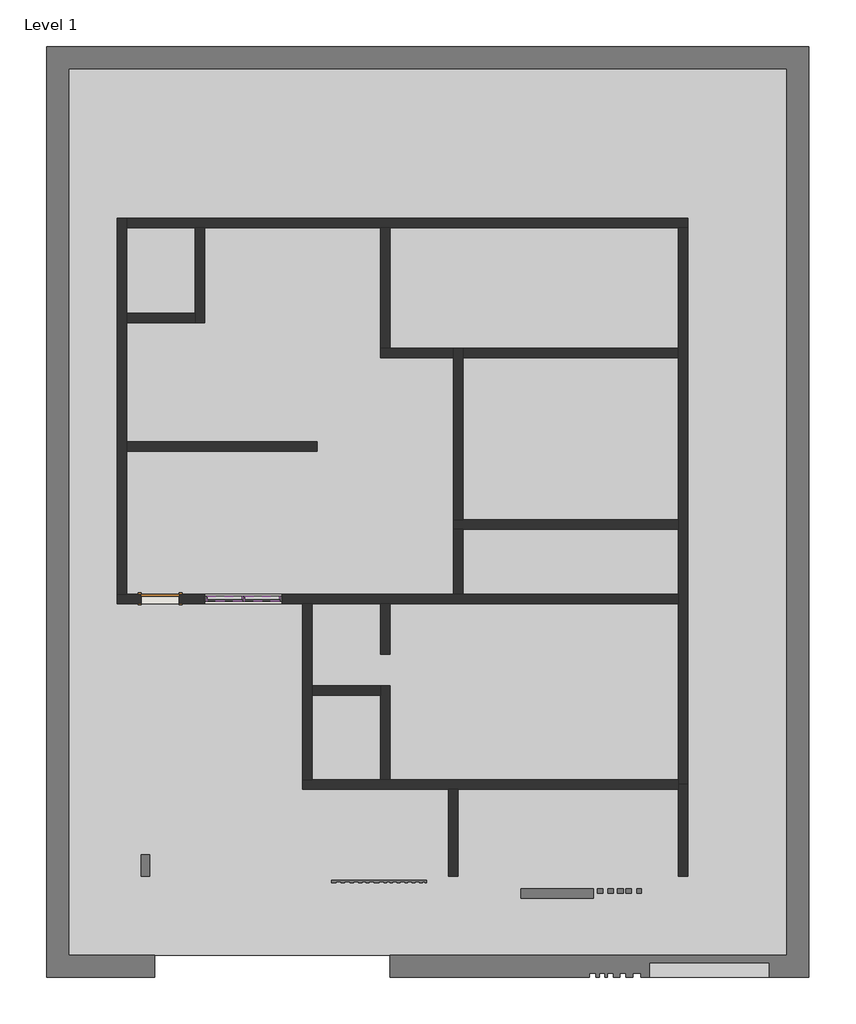
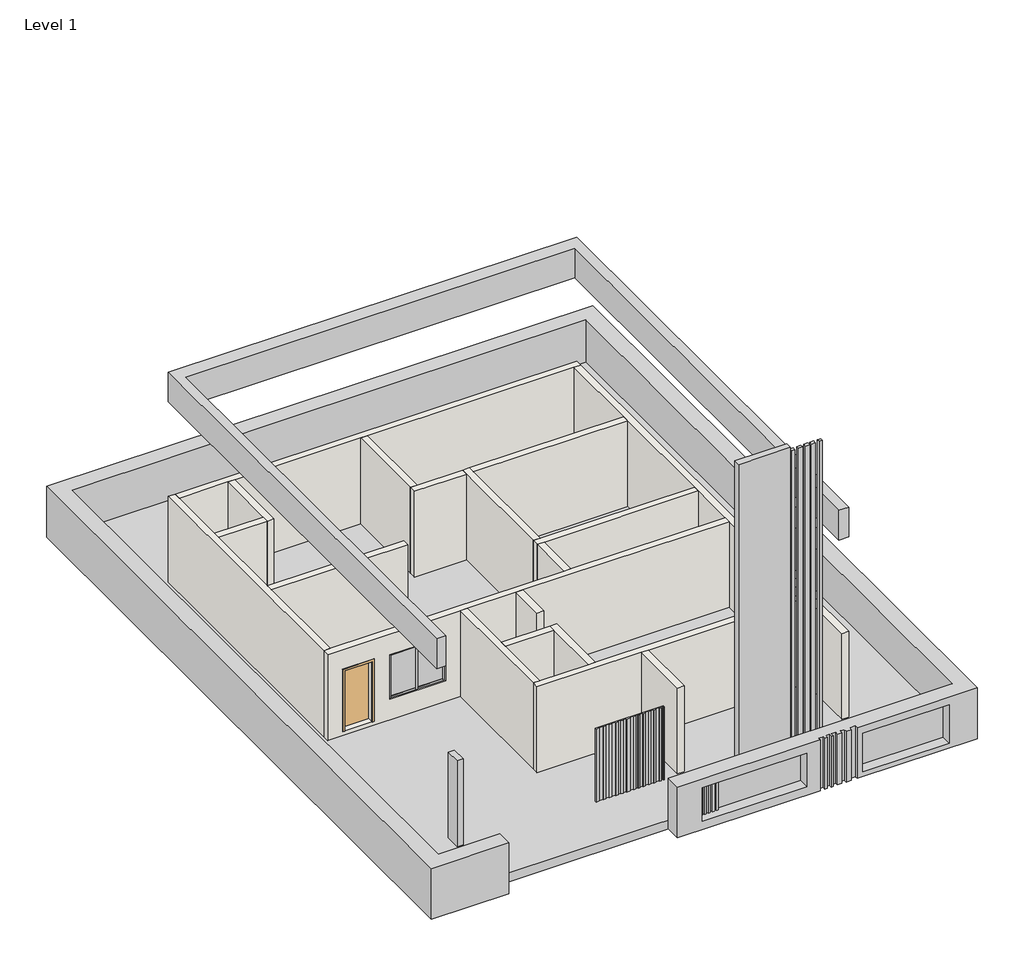
# One storey: 20 walls, 7 members, 3 proxies, 2 plates, 1 door.
"""IFC4 building model written with IfcOpenShell, lengths in millimetres."""

from ifc_helpers import new_model, si_unit, origin, origin_with_axes, place, context, project, spatial, polyline, outline, extrude, faceted_brep, transform, mapped, element, save
from components import generic_models_1_generic_models_1_f562e270, generic_models_2_generic_models_2_9e54925f, generic_models_3_generic_models_3_60b2bde9, door_a90ba1ad, member_86adc6a2, member_ef177d9f, member_d616553b, system_panel_glazed_f96bbed7

model = new_model("IFC4")

# Units and contexts
model_context = context("Model", 3, world=origin())
ifc_project = project(units=[si_unit("LENGTHUNIT", "METRE", prefix="MILLI")], contexts=[model_context])

# Site, building, storey
site = spatial("IfcSite", under=ifc_project)
building = spatial("IfcBuilding", under=site)
storey = spatial("IfcBuildingStorey", under=building, Name="Level 1", Elevation=0.0)

# Proxies
placement = place(None, origin())
generic_models_1_generic_models_1_shape = generic_models_1_generic_models_1_f562e270(model_context)
element("IfcBuildingElementProxy", 1, Name="Generic Models 1 : Generic Models 1", ObjectType="Generic Models 1 : Generic Models 1", at=placement, inside=storey, context=model_context, shape_type="MappedRepresentation", body=[
    mapped(generic_models_1_generic_models_1_shape, transform((0.0, 0.0, 0.0), x_axis=(1.0, 0.0, 0.0), y_axis=(0.0, 1.0, 0.0), z_axis=(0.0, 0.0, 1.0))),
])
generic_models_2_generic_models_2_shape = generic_models_2_generic_models_2_9e54925f(model_context)
element("IfcBuildingElementProxy", 2, Name="Generic Models 2 : Generic Models 2", ObjectType="Generic Models 2 : Generic Models 2", at=placement, inside=storey, context=model_context, shape_type="MappedRepresentation", body=[
    mapped(generic_models_2_generic_models_2_shape, transform((0.0, 0.0, 0.0), x_axis=(1.0, 0.0, 0.0), y_axis=(0.0, 1.0, 0.0), z_axis=(0.0, 0.0, 1.0))),
])
generic_models_3_generic_models_3_shape = generic_models_3_generic_models_3_60b2bde9(model_context)
element("IfcBuildingElementProxy", 3, Name="Generic Models 3 : Generic Models 3", ObjectType="Generic Models 3 : Generic Models 3", at=placement, inside=storey, context=model_context, shape_type="MappedRepresentation", body=[
    mapped(generic_models_3_generic_models_3_shape, transform((0.0, 0.0, 0.0), x_axis=(1.0, 0.0, 0.0), y_axis=(0.0, 1.0, 0.0), z_axis=(0.0, 0.0, 1.0))),
])

# Door
door_shape = door_a90ba1ad(model_context)
element("IfcDoor", 4, ObjectType="Single-Flush : 36\" x 84\"", at=placement, inside=storey, context=model_context, shape_type="MappedRepresentation", body=[
    mapped(door_shape, transform((-16900.3047537, -14441.5428796, 152.4), x_axis=(-1.0, 0.0, 0.0), y_axis=(0.0, -1.0, 0.0), z_axis=(0.0, 0.0, 1.0))),
])

# Members
member_shape = member_86adc6a2(model_context)
element("IfcMember", 5, ObjectType="Rectangular Mullion : 2.5\" x 5\" rectangular", at=placement, inside=storey, context=model_context, shape_type="MappedRepresentation", body=[
    mapped(member_shape, transform((-14868.3047537, -14441.5428796, 2302.9490585), x_axis=(0.0, 0.0, 1.0), y_axis=(0.0, 1.0, 0.0), z_axis=(-1.0, 0.0, 0.0))),
])
element("IfcMember", 6, ObjectType="Rectangular Mullion : 2.5\" x 5\" rectangular", at=placement, inside=storey, context=model_context, shape_type="MappedRepresentation", body=[
    mapped(member_shape, transform((-15770.0047537, -14441.5428796, 2302.9490585), x_axis=(0.0, 0.0, 1.0), y_axis=(0.0, 1.0, 0.0), z_axis=(-1.0, 0.0, 0.0))),
])
member_2_shape = member_ef177d9f(model_context)
element("IfcMember", 7, ObjectType="Rectangular Mullion : 2.5\" x 5\" rectangular", at=placement, inside=storey, context=model_context, shape_type="MappedRepresentation", body=[
    mapped(member_2_shape, transform((-14900.0547537, -14441.5428796, 726.5200737), x_axis=(-1.0, 0.0, 0.0), y_axis=(0.0, 1.0, 0.0), z_axis=(0.0, 0.0, -1.0))),
])
element("IfcMember", 8, ObjectType="Rectangular Mullion : 2.5\" x 5\" rectangular", at=placement, inside=storey, context=model_context, shape_type="MappedRepresentation", body=[
    mapped(member_shape, transform((-14931.8047537, -14441.5428796, 726.5200737), x_axis=(0.0, 0.0, -1.0), y_axis=(0.0, 1.0, 0.0), z_axis=(1.0, 0.0, 0.0))),
])
element("IfcMember", 9, ObjectType="Rectangular Mullion : 2.5\" x 5\" rectangular", at=placement, inside=storey, context=model_context, shape_type="MappedRepresentation", body=[
    mapped(member_shape, transform((-14030.1047537, -14441.5428796, 726.5200737), x_axis=(0.0, 0.0, -1.0), y_axis=(0.0, 1.0, 0.0), z_axis=(1.0, 0.0, 0.0))),
])
member_3_shape = member_d616553b(model_context)
element("IfcMember", 10, ObjectType="Rectangular Mullion : 2.5\" x 5\" rectangular", at=placement, inside=storey, context=model_context, shape_type="MappedRepresentation", body=[
    mapped(member_3_shape, transform((-13966.6047537, -14441.5428796, 2302.9490585), x_axis=(1.0, 0.0, 0.0), y_axis=(0.0, 1.0, 0.0), z_axis=(0.0, 0.0, 1.0))),
])
element("IfcMember", 11, ObjectType="Rectangular Mullion : 2.5\" x 5\" rectangular", at=placement, inside=storey, context=model_context, shape_type="MappedRepresentation", body=[
    mapped(member_3_shape, transform((-15833.5047537, -14441.5428796, 726.5200737), x_axis=(-1.0, 0.0, 0.0), y_axis=(0.0, 1.0, 0.0), z_axis=(0.0, 0.0, -1.0))),
])

# Plates
system_panel_glazed_shape = system_panel_glazed_f96bbed7(model_context)
element("IfcPlate", 12, ObjectType="System Panel : Glazed", at=placement, inside=storey, context=model_context, shape_type="MappedRepresentation", body=[
    mapped(system_panel_glazed_shape, transform((-14449.2047537, -14441.5428796, 790.0200737), x_axis=(-1.0, 0.0, 0.0), y_axis=(0.0, -1.0, 0.0), z_axis=(0.0, 0.0, 1.0))),
])
element("IfcPlate", 13, ObjectType="System Panel : Glazed", at=placement, inside=storey, context=model_context, shape_type="MappedRepresentation", body=[
    mapped(system_panel_glazed_shape, transform((-15350.9047537, -14441.5428796, 790.0200737), x_axis=(-1.0, 0.0, 0.0), y_axis=(0.0, -1.0, 0.0), z_axis=(0.0, 0.0, 1.0))),
])

# Walls
element("IfcWall", 14, ObjectType="9\"", at=placement, inside=storey, context=model_context, shape_type="Brep", body=[
    faceted_brep([(-17929.0047537, -14555.8428796, 0.0), (-13471.3047537, -14555.8428796, 0.0), (-13242.7047537, -14555.8428796, 0.0), (-11604.4047537, -14555.8428796, 0.0), (-11375.8047537, -14555.8428796, 0.0), (-4441.6047537, -14555.8428796, 0.0), (-4441.6047537, -14555.8428796, 3048.0), (-11375.8047537, -14555.8428796, 3048.0), (-11604.4047537, -14555.8428796, 3048.0), (-13242.7047537, -14555.8428796, 3048.0), (-13471.3047537, -14555.8428796, 3048.0), (-17929.0047537, -14555.8428796, 3048.0), (-16443.1047537, -14555.8428796, 152.4), (-17357.5047537, -14555.8428796, 152.4), (-17357.5047537, -14555.8428796, 2286.0), (-16443.1047537, -14555.8428796, 2286.0), (-13966.6047537, -14555.8428796, 2302.9490585), (-13966.6047537, -14555.8428796, 726.5200737), (-15833.5047537, -14555.8428796, 726.5200737), (-15833.5047537, -14555.8428796, 2302.9490585), (-4441.6047537, -14327.2428796, 0.0), (-9623.2047537, -14327.2428796, 0.0), (-9851.8047537, -14327.2428796, 0.0), (-17700.4047537, -14327.2428796, 0.0), (-17929.0047537, -14327.2428796, 0.0), (-17929.0047537, -14327.2428796, 3048.0), (-17700.4047537, -14327.2428796, 3048.0), (-9851.8047537, -14327.2428796, 3048.0), (-9623.2047537, -14327.2428796, 3048.0), (-4441.6047537, -14327.2428796, 3048.0), (-17357.5047537, -14327.2428796, 152.4), (-16443.1047537, -14327.2428796, 152.4), (-16443.1047537, -14327.2428796, 2286.0), (-17357.5047537, -14327.2428796, 2286.0), (-13966.6047537, -14327.2428796, 726.5200737), (-13966.6047537, -14327.2428796, 2302.9490585), (-15833.5047537, -14327.2428796, 2302.9490585), (-15833.5047537, -14327.2428796, 726.5200737)], [[[0, 1, 2, 3, 4, 5, 6, 7, 8, 9, 10, 11], [12, 13, 14, 15], [16, 17, 18, 19]], [[20, 21, 22, 23, 24, 25, 26, 27, 28, 29], [30, 31, 32, 33], [34, 35, 36, 37]], [[5, 4, 3, 2, 1, 0, 24, 23, 22, 21, 20]], [[11, 10, 9, 8, 7, 6, 29, 28, 27, 26, 25]], [[0, 11, 25, 24]], [[6, 5, 20, 29]], [[13, 12, 31, 30]], [[14, 13, 30, 33]], [[15, 14, 33, 32]], [[12, 15, 32, 31]], [[34, 17, 16, 35]], [[35, 16, 19, 36]], [[36, 19, 18, 37]], [[17, 34, 37, 18]]]),
])
element("IfcWall", 15, ObjectType="9\"", at=placement, inside=storey, context=model_context, shape_type="Brep", body=[
    faceted_brep([(-17700.4047537, -14327.2428796, 0.0), (-17700.4047537, -10898.2428796, 0.0), (-17700.4047537, -10669.6428796, 0.0), (-17700.4047537, -7812.1428796, 0.0), (-17700.4047537, -7583.5428796, 0.0), (-17700.4047537, -5526.1428796, 0.0), (-17700.4047537, -5297.5428796, 0.0), (-17700.4047537, -5297.5428796, 3048.0), (-17700.4047537, -5526.1428796, 3048.0), (-17700.4047537, -7583.5428796, 3048.0), (-17700.4047537, -7812.1428796, 3048.0), (-17700.4047537, -10669.6428796, 3048.0), (-17700.4047537, -10898.2428796, 3048.0), (-17700.4047537, -14327.2428796, 3048.0), (-17929.0047537, -14327.2428796, 0.0), (-17929.0047537, -14327.2428796, 3048.0), (-17929.0047537, -5297.5428796, 3048.0), (-17929.0047537, -5297.5428796, 0.0)], [[[0, 1, 2, 3, 4, 5, 6, 7, 8, 9, 10, 11, 12, 13]], [[14, 15, 16, 17]], [[6, 5, 4, 3, 2, 1, 0, 14, 17]], [[13, 12, 11, 10, 9, 8, 7, 16, 15]], [[0, 13, 15, 14]], [[7, 6, 17, 16]]]),
])
element("IfcWall", 16, ObjectType="9\"", at=placement, inside=storey, context=model_context, shape_type="Brep", body=[
    faceted_brep([(-17700.4047537, -5526.1428796, 0.0), (-16062.1047537, -5526.1428796, 0.0), (-15833.5047537, -5526.1428796, 0.0), (-11604.4047537, -5526.1428796, 0.0), (-11375.8047537, -5526.1428796, 0.0), (-4441.6047537, -5526.1428796, 0.0), (-4213.0047537, -5526.1428796, 0.0), (-4213.0047537, -5526.1428796, 3048.0), (-4441.6047537, -5526.1428796, 3048.0), (-11375.8047537, -5526.1428796, 3048.0), (-11604.4047537, -5526.1428796, 3048.0), (-15833.5047537, -5526.1428796, 3048.0), (-16062.1047537, -5526.1428796, 3048.0), (-17700.4047537, -5526.1428796, 3048.0), (-17700.4047537, -5297.5428796, 0.0), (-17700.4047537, -5297.5428796, 3048.0), (-4213.0047537, -5297.5428796, 3048.0), (-4213.0047537, -5297.5428796, 0.0)], [[[0, 1, 2, 3, 4, 5, 6, 7, 8, 9, 10, 11, 12, 13]], [[14, 15, 16, 17]], [[6, 5, 4, 3, 2, 1, 0, 14, 17]], [[13, 12, 11, 10, 9, 8, 7, 16, 15]], [[0, 13, 15, 14]], [[7, 6, 17, 16]]]),
])
element("IfcWall", 17, ObjectType="9\"", at=placement, inside=storey, context=model_context, shape_type="Brep", body=[
    faceted_brep([(-4441.6047537, -5526.1428796, 0.0), (-4441.6047537, -8421.7428796, 0.0), (-4441.6047537, -8650.3428796, 0.0), (-4441.6047537, -12536.5428796, 0.0), (-4441.6047537, -12765.1428796, 0.0), (-4441.6047537, -14327.2428796, 0.0), (-4441.6047537, -14555.8428796, 0.0), (-4441.6047537, -18784.9428796, 0.0), (-4441.6047537, -18899.2428796, 0.0), (-4441.6047537, -18899.2428796, 3048.0), (-4441.6047537, -18784.9428796, 3048.0), (-4441.6047537, -14555.8428796, 3048.0), (-4441.6047537, -14327.2428796, 3048.0), (-4441.6047537, -12765.1428796, 3048.0), (-4441.6047537, -12536.5428796, 3048.0), (-4441.6047537, -8650.3428796, 3048.0), (-4441.6047537, -8421.7428796, 3048.0), (-4441.6047537, -5526.1428796, 3048.0), (-4213.0047537, -5526.1428796, 0.0), (-4213.0047537, -5526.1428796, 3048.0), (-4213.0047537, -18899.2428796, 3048.0), (-4213.0047537, -18899.2428796, 0.0)], [[[0, 1, 2, 3, 4, 5, 6, 7, 8, 9, 10, 11, 12, 13, 14, 15, 16, 17]], [[18, 19, 20, 21]], [[8, 7, 6, 5, 4, 3, 2, 1, 0, 18, 21]], [[9, 8, 21, 20]], [[17, 16, 15, 14, 13, 12, 11, 10, 9, 20, 19]], [[0, 17, 19, 18]]]),
])
element("IfcWall", 18, ObjectType="9\"", at=placement, inside=storey, context=model_context, shape_type="Brep", body=[
    faceted_brep([(-4441.6047537, -18784.9428796, 0.0), (-11375.8047537, -18784.9428796, 0.0), (-11604.4047537, -18784.9428796, 0.0), (-13242.7047537, -18784.9428796, 0.0), (-13471.3047537, -18784.9428796, 0.0), (-13471.3047537, -18784.9428796, 3048.0), (-13242.7047537, -18784.9428796, 3048.0), (-11604.4047537, -18784.9428796, 3048.0), (-11375.8047537, -18784.9428796, 3048.0), (-4441.6047537, -18784.9428796, 3048.0), (-4441.6047537, -19013.5428796, 0.0), (-4441.6047537, -19013.5428796, 3048.0), (-9737.5047537, -19013.5428796, 3048.0), (-9966.1047537, -19013.5428796, 3048.0), (-13471.3047537, -19013.5428796, 3048.0), (-13471.3047537, -19013.5428796, 0.0), (-9966.1047537, -19013.5428796, 0.0), (-9737.5047537, -19013.5428796, 0.0), (-4441.6047537, -18899.2428796, 0.0), (-4441.6047537, -18899.2428796, 3048.0)], [[[0, 1, 2, 3, 4, 5, 6, 7, 8, 9]], [[10, 11, 12, 13, 14, 15, 16, 17]], [[4, 3, 2, 1, 0, 18, 10, 17, 16, 15]], [[9, 8, 7, 6, 5, 14, 13, 12, 11, 19]], [[5, 4, 15, 14]], [[0, 9, 19, 11, 10, 18]]]),
])
element("IfcWall", 19, ObjectType="9\"", at=placement, inside=storey, context=model_context, shape_type="Brep", body=[
    faceted_brep([(-13242.7047537, -18784.9428796, 0.0), (-13242.7047537, -16765.6428796, 0.0), (-13242.7047537, -16537.0428796, 0.0), (-13242.7047537, -14555.8428796, 0.0), (-13242.7047537, -14555.8428796, 3048.0), (-13242.7047537, -16537.0428796, 3048.0), (-13242.7047537, -16765.6428796, 3048.0), (-13242.7047537, -18784.9428796, 3048.0), (-13471.3047537, -18784.9428796, 0.0), (-13471.3047537, -18784.9428796, 3048.0), (-13471.3047537, -14555.8428796, 3048.0), (-13471.3047537, -14555.8428796, 0.0)], [[[0, 1, 2, 3, 4, 5, 6, 7]], [[8, 9, 10, 11]], [[3, 2, 1, 0, 8, 11]], [[7, 6, 5, 4, 10, 9]], [[0, 7, 9, 8]], [[4, 3, 11, 10]]]),
])
element("IfcWall", 20, ObjectType="9\"", at=placement, inside=storey, context=model_context, shape_type="SweptSolid", body=[
    extrude(outline(polyline([(-11604.4047537, -15775.0428796), (-11604.4047537, -14555.8428796), (-11375.8047537, -14555.8428796), (-11375.8047537, -15775.0428796), (-11604.4047537, -15775.0428796)])), origin_with_axes(), (0.0, 0.0, 1.0), 3048.0),
])
element("IfcWall", 21, ObjectType="9\"", at=placement, inside=storey, context=model_context, shape_type="Brep", body=[
    faceted_brep([(-11604.4047537, -16537.0428796, 0.0), (-11604.4047537, -16765.6428796, 0.0), (-11604.4047537, -18784.9428796, 0.0), (-11604.4047537, -18784.9428796, 3048.0), (-11604.4047537, -16765.6428796, 3048.0), (-11604.4047537, -16537.0428796, 3048.0), (-11375.8047537, -16537.0428796, 0.0), (-11375.8047537, -16537.0428796, 3048.0), (-11375.8047537, -18784.9428796, 3048.0), (-11375.8047537, -18784.9428796, 0.0)], [[[0, 1, 2, 3, 4, 5]], [[6, 7, 8, 9]], [[2, 1, 0, 6, 9]], [[5, 4, 3, 8, 7]], [[3, 2, 9, 8]], [[0, 5, 7, 6]]]),
])
element("IfcWall", 22, ObjectType="9\"", at=placement, inside=storey, context=model_context, shape_type="SweptSolid", body=[
    extrude(outline(polyline([(-13242.7047537, -16537.0428796), (-11604.4047537, -16537.0428796), (-11604.4047537, -16765.6428796), (-13242.7047537, -16765.6428796), (-13242.7047537, -16537.0428796)])), origin_with_axes(), (0.0, 0.0, 1.0), 3048.0),
])
element("IfcWall", 23, ObjectType="9\"", at=placement, inside=storey, context=model_context, shape_type="Brep", body=[
    faceted_brep([(-4441.6047537, -12536.5428796, 0.0), (-9623.2047537, -12536.5428796, 0.0), (-9851.8047537, -12536.5428796, 0.0), (-9851.8047537, -12536.5428796, 3048.0), (-9623.2047537, -12536.5428796, 3048.0), (-4441.6047537, -12536.5428796, 3048.0), (-4441.6047537, -12765.1428796, 0.0), (-4441.6047537, -12765.1428796, 3048.0), (-9623.2047537, -12765.1428796, 3048.0), (-9851.8047537, -12765.1428796, 3048.0), (-9851.8047537, -12765.1428796, 0.0), (-9623.2047537, -12765.1428796, 0.0)], [[[0, 1, 2, 3, 4, 5]], [[6, 7, 8, 9, 10, 11]], [[2, 1, 0, 6, 11, 10]], [[5, 4, 3, 9, 8, 7]], [[0, 5, 7, 6]], [[3, 2, 10, 9]]]),
])
element("IfcWall", 24, ObjectType="9\"", at=placement, inside=storey, context=model_context, shape_type="SweptSolid", body=[
    extrude(outline(polyline([(-9851.8047537, -14327.2428796), (-9851.8047537, -12765.1428796), (-9623.2047537, -12765.1428796), (-9623.2047537, -14327.2428796), (-9851.8047537, -14327.2428796)])), origin_with_axes(), (0.0, 0.0, 1.0), 3048.0),
])
element("IfcWall", 25, ObjectType="9\"", at=placement, inside=storey, context=model_context, shape_type="Brep", body=[
    faceted_brep([(-9623.2047537, -12536.5428796, 0.0), (-9623.2047537, -8650.3428796, 0.0), (-9623.2047537, -8421.7428796, 0.0), (-9623.2047537, -8421.7428796, 3048.0), (-9623.2047537, -8650.3428796, 3048.0), (-9623.2047537, -12536.5428796, 3048.0), (-9851.8047537, -12536.5428796, 0.0), (-9851.8047537, -12536.5428796, 3048.0), (-9851.8047537, -8650.3428796, 3048.0), (-9851.8047537, -8421.7428796, 3048.0), (-9851.8047537, -8421.7428796, 0.0), (-9851.8047537, -8650.3428796, 0.0)], [[[0, 1, 2, 3, 4, 5]], [[6, 7, 8, 9, 10, 11]], [[2, 1, 0, 6, 11, 10]], [[5, 4, 3, 9, 8, 7]], [[0, 5, 7, 6]], [[3, 2, 10, 9]]]),
])
element("IfcWall", 26, ObjectType="9\"", at=placement, inside=storey, context=model_context, shape_type="SweptSolid", body=[
    extrude(outline(polyline([(-4441.6047537, -8650.3428796), (-9623.2047537, -8650.3428796), (-9623.2047537, -8421.7428796), (-4441.6047537, -8421.7428796), (-4441.6047537, -8650.3428796)])), origin_with_axes(), (0.0, 0.0, 1.0), 3048.0),
])
element("IfcWall", 27, ObjectType="9\"", at=placement, inside=storey, context=model_context, shape_type="Brep", body=[
    faceted_brep([(-9851.8047537, -8421.7428796, 0.0), (-11375.8047537, -8421.7428796, 0.0), (-11604.4047537, -8421.7428796, 0.0), (-11604.4047537, -8421.7428796, 3048.0), (-11375.8047537, -8421.7428796, 3048.0), (-9851.8047537, -8421.7428796, 3048.0), (-9851.8047537, -8650.3428796, 0.0), (-9851.8047537, -8650.3428796, 3048.0), (-11604.4047537, -8650.3428796, 3048.0), (-11604.4047537, -8650.3428796, 0.0)], [[[0, 1, 2, 3, 4, 5]], [[6, 7, 8, 9]], [[2, 1, 0, 6, 9]], [[5, 4, 3, 8, 7]], [[0, 5, 7, 6]], [[3, 2, 9, 8]]]),
])
element("IfcWall", 28, ObjectType="9\"", at=placement, inside=storey, context=model_context, shape_type="SweptSolid", body=[
    extrude(outline(polyline([(-11375.8047537, -5526.1428796), (-11375.8047537, -8421.7428796), (-11604.4047537, -8421.7428796), (-11604.4047537, -5526.1428796), (-11375.8047537, -5526.1428796)])), origin_with_axes(), (0.0, 0.0, 1.0), 3048.0),
])
element("IfcWall", 29, ObjectType="9\"", at=placement, inside=storey, context=model_context, shape_type="Brep", body=[
    faceted_brep([(-16062.1047537, -5526.1428796, 0.0), (-16062.1047537, -7583.5428796, 0.0), (-16062.1047537, -7812.1428796, 0.0), (-16062.1047537, -7812.1428796, 3048.0), (-16062.1047537, -7583.5428796, 3048.0), (-16062.1047537, -5526.1428796, 3048.0), (-15833.5047537, -5526.1428796, 0.0), (-15833.5047537, -5526.1428796, 3048.0), (-15833.5047537, -7812.1428796, 3048.0), (-15833.5047537, -7812.1428796, 0.0)], [[[0, 1, 2, 3, 4, 5]], [[6, 7, 8, 9]], [[2, 1, 0, 6, 9]], [[5, 4, 3, 8, 7]], [[0, 5, 7, 6]], [[3, 2, 9, 8]]]),
])
element("IfcWall", 30, ObjectType="9\"", at=placement, inside=storey, context=model_context, shape_type="SweptSolid", body=[
    extrude(outline(polyline([(-17700.4047537, -7583.5428796), (-16062.1047537, -7583.5428796), (-16062.1047537, -7812.1428796), (-17700.4047537, -7812.1428796), (-17700.4047537, -7583.5428796)])), origin_with_axes(), (0.0, 0.0, 1.0), 3048.0),
])
element("IfcWall", 31, ObjectType="9\"", at=placement, inside=storey, context=model_context, shape_type="SweptSolid", body=[
    extrude(outline(polyline([(-13128.4047537, -10898.2428796), (-17700.4047537, -10898.2428796), (-17700.4047537, -10669.6428796), (-13128.4047537, -10669.6428796), (-13128.4047537, -10898.2428796)])), origin_with_axes(), (0.0, 0.0, 1.0), 3048.0),
])
element("IfcWall", 32, ObjectType="9\"", at=placement, inside=storey, context=model_context, shape_type="SweptSolid", body=[
    extrude(outline(polyline([(-9966.1047537, -21109.0428796), (-9966.1047537, -19013.5428796), (-9737.5047537, -19013.5428796), (-9737.5047537, -21109.0428796), (-9966.1047537, -21109.0428796)])), origin_with_axes(), (0.0, 0.0, 1.0), 3048.0),
])
element("IfcWall", 33, ObjectType="9\"", at=placement, inside=storey, context=model_context, shape_type="Brep", body=[
    faceted_brep([(-4213.0047537, -21109.0428796, 0.0), (-4213.0047537, -18899.2428796, 0.0), (-4213.0047537, -18899.2428796, 3048.0), (-4213.0047537, -21109.0428796, 3048.0), (-4441.6047537, -21109.0428796, 0.0), (-4441.6047537, -21109.0428796, 3048.0), (-4441.6047537, -19013.5428796, 3048.0), (-4441.6047537, -18899.2428796, 3048.0), (-4441.6047537, -18899.2428796, 0.0), (-4441.6047537, -19013.5428796, 0.0)], [[[0, 1, 2, 3]], [[4, 5, 6, 7, 8, 9]], [[1, 0, 4, 9, 8]], [[2, 1, 8, 7]], [[3, 2, 7, 6, 5]], [[0, 3, 5, 4]]]),
])

save(model, "model.ifc")

# Revit data of these elements
# Type "Single-Flush : 36\" x 84\""
#   Type Mark = "1"
#   Construction Type Id = "MDOOR"
#   Assembly Code = "C1020"
#   Analytic Construction = "Metal"
#   Thickness = 0' - 2"
#   Heat Transfer Coefficient (U) = 0.651978 BTU/(h·ft²·°F)
#   Height = 7' - 0"
#   Trim Projection Ext = 0' - 1"
#   Trim Projection Int = 0' - 1"
#   Trim Width = 0' - 3"
#   Width = 3' - 0"
#   Define Thermal Properties by = 1
#   Define Thermal Properties by = 1
#   Door Material = Door - Panel
#   Frame Material = Door - Frame
#   Visual Light Transmittance = 0
#   Solar Heat Gain Coefficient = 0
#   Function = (empty or 0)
#   Wall Closure = (empty or 0)
# Type "Rectangular Mullion : 2.5\" x 5\" rectangular"
#   built-in parameter 1007304 = 0.416667 (stored number, unit not read)
#   built-in parameter 1007301 = 0.104167 (stored number, unit not read)
#   built-in parameter 1007300 = 0.104167 (stored number, unit not read)
# Type "System Panel : Glazed"
#   Construction Type Id = "GSP4R"
#   Analytic Construction = "1/8 in Pilkington single glazing"
#   Visual Light Transmittance = 0.9
#   Solar Heat Gain Coefficient = 0.86
#   Heat Transfer Coefficient (U) = 1.18115 BTU/(h·ft²·°F)
#   Define Thermal Properties by = 1
# Type "9\""
#   Assembly Code = "B2010"
#   Layers, outside or top first: 0' - 9" no material (function 1)
# Element 1 (IfcBuildingElementProxy, "Generic Models 1 : Generic Models 1")
#   Phase Created = New Construction
# Element 2 (IfcBuildingElementProxy, "Generic Models 2 : Generic Models 2")
#   Phase Created = New Construction
# Element 3 (IfcBuildingElementProxy, "Generic Models 3 : Generic Models 3")
#   Phase Created = New Construction
# Element 4 (IfcDoor, "Single-Flush : 36\" x 84\"")
#   Phase Created = New Construction
#   Materials on its faces: "Door - Frame", "Door - Panel"
# Elements 5, 6, 7, 8, 9, 10, 11 (IfcMember, "Rectangular Mullion : 2.5\" x 5\" rectangular")
#   Phase Created = New Construction
#   Materials on its faces: "Aluminum"
# Elements 12, 13 (IfcPlate, "System Panel : Glazed")
#   Phase Created = New Construction
#   Materials on its faces: "Glass"
# Elements 14, 15, 16, 17, 18, 19, 20, 21, 22, 23, 24, 25, 26, 27, 28, 29, 30, 31, 32, 33 (IfcWall, "9\"")
#   Top Offset = 0' - 0"
#   Base Offset = 0' - 0"
#   Unconnected Height = 10' - 0"
#   wall height = 10' - 0"
#   Phase Created = New Construction
#   Base Constraint = Level 1
#   Materials on its faces: "Default Wall"
# Materials
#   "Door - Panel": class "Wood", colour RGB 210 159 95, transparency 0, Cost = 0
#   "Door - Frame": colour RGB 118 70 51, transparency 0, Cost = 0
#   "Aluminum": class "Metal", colour RGB 247 247 247, transparency 0, Description = "Aluminum 6061", Cost = 0
#   "Glass": class "Glass", colour RGB 0 128 192, transparency 0.75, Description = "Soda Lime Glass", Cost = 0
#   "Default Wall": colour RGB 128 128 128, transparency 0, Cost = 0
